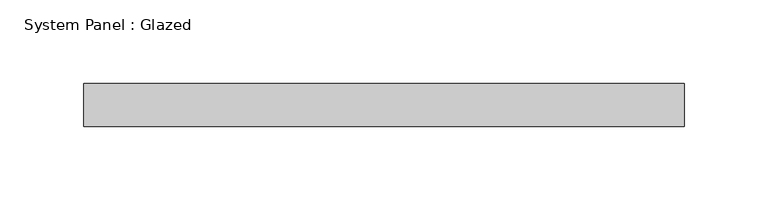
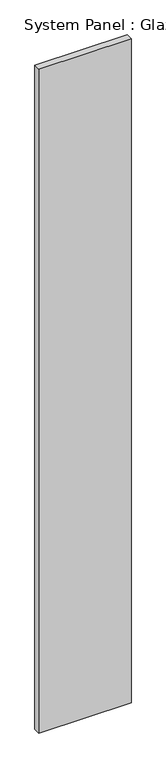
"""IFC4 building model written with IfcOpenShell, lengths in millimetres: plate geometry, System Panel : Glazed."""

from ifc_helpers import new_model, si_unit, origin, origin_with_axes, place, context, project, spatial, polyline, outline, extrude, source, transform, mapped, element, save


def system_panel_glazed_6096bcca(model_context):
    return source(origin(), model_context, "Body", "SweptSolid", [
        extrude(outline(polyline([(178.8583333, 19.05), (-178.8583333, 19.05), (-178.8583333, 44.45), (178.8583333, 44.45), (178.8583333, 19.05)])), origin_with_axes(), (0.0, 0.0, 1.0), 2719.788773),
    ])


if __name__ == "__main__":
    model = new_model("IFC4")
    model_context = context("Model", 3, world=origin())
    ifc_project = project(units=[si_unit("LENGTHUNIT", "METRE", prefix="MILLI")], contexts=[model_context])
    site = spatial("IfcSite", under=ifc_project)
    building = spatial("IfcBuilding", under=site)
    placement = place(None, origin())
    system_panel_glazed_shape = system_panel_glazed_6096bcca(model_context)
    element("IfcPlate", 1, ObjectType="System Panel : Glazed", at=placement, inside=building, context=model_context, shape_type="MappedRepresentation", body=[
        mapped(system_panel_glazed_shape, transform((0.0, 0.0, 0.0), x_axis=(1.0, 0.0, 0.0), y_axis=(0.0, 1.0, 0.0), z_axis=(0.0, 0.0, 1.0))),
    ])
    save(model, "model.ifc")

# Revit data of these elements
# Type "System Panel : Glazed"
#   Construction Type Id = "GSP4R"
#   Analytic Construction = "1/8 in Pilkington single glazing"
#   Visual Light Transmittance = 0.9
#   Solar Heat Gain Coefficient = 0.86
#   Heat Transfer Coefficient (U) = 1.18115 BTU/(h·ft²·°F)
# Element 1 (IfcPlate, "System Panel : Glazed")
#   Materials on its faces: "Glass"
# Materials
#   "Glass": class "Glass", colour RGB 0 128 192, transparency 0.75, Description = "Soda Lime Glass", Cost = 0
